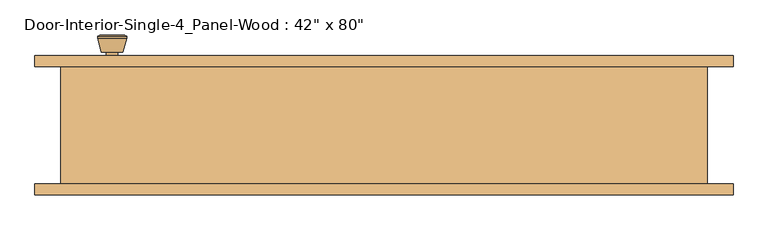
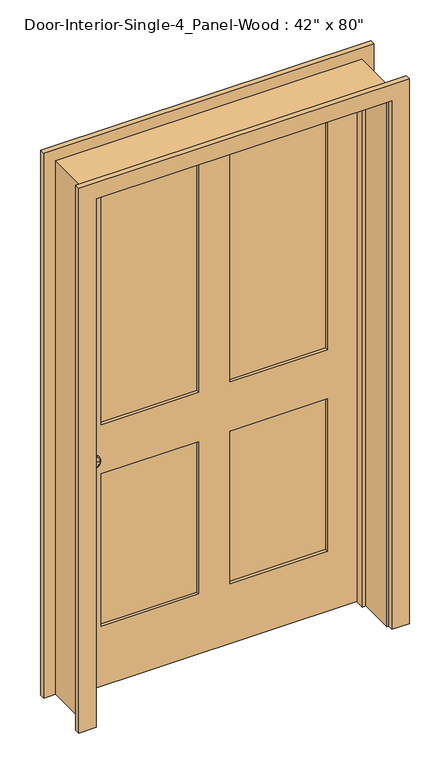
"""IFC4 building model written with IfcOpenShell, lengths in millimetres: door geometry."""

from ifc_helpers import new_model, si_unit, point, frame, frame_2d, origin, place, context, project, spatial, polyline, circle_curve, trimmed, segment, composite_curve, outline, extrude, faceted_brep, source, transform, mapped, element, save
from ifc_brep_helpers import plane_surface, cylinder_surface, revolved_surface, advanced_brep


def door_63baf7d0(model_context):
    return source(origin(), model_context, "Body", "SolidModel", [
        advanced_brep(
        [(-469.9, 57.5, 914.4), (-459.9, 57.5, 914.4), (-479.9, 57.5, 914.4), (-449.4241324, 8.5, 914.4), (-469.9, 8.5, 914.4), (-490.3758676, 8.5, 914.4), (-444.9, 10.3278681, 914.4), (-494.9, 10.3278681, 914.4), (-444.9, 13.7915463, 914.4), (-494.9, 13.7915463, 914.4), (-451.263764, 38.5, 914.4), (-488.536236, 38.5, 914.4), (-459.9, 38.5, 914.4), (-479.9, 38.5, 914.4)],
        [
            (0, 1),
            (1, 2, circle_curve(frame((-469.9, 57.5, 914.4), z_axis=(0.0, 1.0, 0.0), x_axis=(-1.0, 0.0, 0.0)), 10.0)),
            (2, 0),
            (2, 1, circle_curve(frame((-469.9, 57.5, 914.4), z_axis=(0.0, 1.0, 0.0), x_axis=(-1.0, 0.0, 0.0)), 10.0)),
            (3, 4),
            (4, 5),
            (5, 3, circle_curve(frame((-469.9, 8.5, 914.4), z_axis=(0.0, -1.0, 0.0), x_axis=(-1.0, 0.0, 0.0)), 20.4758676)),
            (3, 5, circle_curve(frame((-469.9, 8.5, 914.4), z_axis=(0.0, -1.0, 0.0), x_axis=(-1.0, 0.0, 0.0)), 20.4758676)),
            (6, 3),
            (5, 7),
            (7, 6, circle_curve(frame((-469.9, 10.3278681, 914.4), z_axis=(0.0, -1.0, 0.0), x_axis=(-1.0, 0.0, 0.0)), 25.0)),
            (6, 7, circle_curve(frame((-469.9, 10.3278681, 914.4), z_axis=(0.0, -1.0, 0.0), x_axis=(-1.0, 0.0, 0.0)), 25.0)),
            (8, 6),
            (7, 9),
            (9, 8, circle_curve(frame((-469.9, 13.7915463, 914.4), z_axis=(0.0, -1.0, 0.0), x_axis=(-1.0, 0.0, 0.0)), 25.0)),
            (8, 9, circle_curve(frame((-469.9, 13.7915463, 914.4), z_axis=(0.0, -1.0, 0.0), x_axis=(-1.0, 0.0, 0.0)), 25.0)),
            (10, 8),
            (9, 11),
            (11, 10, circle_curve(frame((-469.9, 38.5, 914.4), z_axis=(0.0, -1.0, 0.0), x_axis=(-1.0, 0.0, 0.0)), 18.636236)),
            (10, 11, circle_curve(frame((-469.9, 38.5, 914.4), z_axis=(0.0, -1.0, 0.0), x_axis=(-1.0, 0.0, 0.0)), 18.636236)),
            (12, 10),
            (11, 13),
            (13, 12, circle_curve(frame((-469.9, 38.5, 914.4), z_axis=(0.0, -1.0, 0.0), x_axis=(-1.0, 0.0, 0.0)), 10.0)),
            (12, 13, circle_curve(frame((-469.9, 38.5, 914.4), z_axis=(0.0, -1.0, 0.0), x_axis=(-1.0, 0.0, 0.0)), 10.0)),
            (1, 12),
            (13, 2),
        ],
        [
            plane_surface(frame((-469.9, 57.5, 914.4), z_axis=(0.0, 1.0, 0.0), x_axis=(-1.0, 0.0, 0.0))),
            plane_surface(frame((-469.9, 8.5, 914.4), z_axis=(0.0, -1.0, 0.0), x_axis=(-1.0, 0.0, 0.0))),
            revolved_surface(polyline([(-490.3758676, 8.5, 914.4), (-494.9, 10.3278681, 914.4)]), (-469.9, 57.5, 914.4), (0.0, 1.0, 0.0)),
            cylinder_surface(frame((-469.9, 57.5, 914.4), z_axis=(0.0, 1.0, 0.0), x_axis=(-1.0, 0.0, 0.0)), 25.0),
            revolved_surface(polyline([(-494.9, 13.7915463, 914.4), (-488.536236, 38.5, 914.4)]), (-469.9, 57.5, 914.4), (0.0, 1.0, 0.0)),
            plane_surface(frame((-469.9, 38.5, 914.4), z_axis=(0.0, 1.0, 0.0), x_axis=(-1.0, 0.0, 0.0))),
            cylinder_surface(frame((-469.9, 57.5, 914.4), z_axis=(0.0, 1.0, 0.0), x_axis=(-1.0, 0.0, 0.0)), 10.0),
        ],
        [
            (0, [[1, 2, 3]]),
            (0, [[-3, 4, -1]]),
            (1, [[5, 6, 7]]),
            (1, [[-6, -5, 8]]),
            (2, [[9, -7, 10, 11]]),
            (2, [[-10, -8, -9, 12]]),
            (3, [[13, -11, 14, 15]]),
            (3, [[-14, -12, -13, 16]]),
            (4, [[17, -15, 18, 19]]),
            (4, [[-18, -16, -17, 20]]),
            (5, [[21, -19, 22, 23]]),
            (5, [[-22, -20, -21, 24]]),
            (6, [[25, -23, 26, -2]]),
            (6, [[-26, -24, -25, -4]]),
        ],
    ),
        extrude(outline(composite_curve([segment(trimmed(circle_curve(frame_2d((914.4, -469.9)), 30.0), [point((914.4, -499.9))], [point((914.4, -439.9))], False, "CARTESIAN"), True, "CONTINUOUS"), segment(trimmed(circle_curve(frame_2d((914.4, -469.9)), 30.0), [point((914.4, -439.9))], [point((914.4, -499.9))], False, "CARTESIAN"), True, "CONTINUOUS")], self_intersect=False)), frame((0.0, 57.5, 0.0), z_axis=(0.0, 1.0, 0.0), x_axis=(0.0, 0.0, 1.0)), (0.0, 0.0, 1.0), 6.0),
        advanced_brep(
        [(-469.9, 104.425, 914.4), (-479.9, 104.425, 914.4), (-459.9, 104.425, 914.4), (-449.4241324, 153.425, 914.4), (-490.3758676, 153.425, 914.4), (-469.9, 153.425, 914.4), (-444.9, 151.5971319, 914.4), (-494.9, 151.5971319, 914.4), (-444.9, 148.1334537, 914.4), (-494.9, 148.1334537, 914.4), (-451.263764, 123.425, 914.4), (-488.536236, 123.425, 914.4), (-459.9, 123.425, 914.4), (-479.9, 123.425, 914.4)],
        [
            (0, 1),
            (1, 2, circle_curve(frame((-469.9, 104.425, 914.4), z_axis=(0.0, -1.0, 0.0), x_axis=(-1.0, 0.0, 0.0)), 10.0)),
            (2, 0),
            (2, 1, circle_curve(frame((-469.9, 104.425, 914.4), z_axis=(0.0, -1.0, 0.0), x_axis=(-1.0, 0.0, 0.0)), 10.0)),
            (3, 4, circle_curve(frame((-469.9, 153.425, 914.4), z_axis=(0.0, 1.0, 0.0), x_axis=(-1.0, 0.0, 0.0)), 20.4758676)),
            (4, 5),
            (5, 3),
            (4, 3, circle_curve(frame((-469.9, 153.425, 914.4), z_axis=(0.0, 1.0, 0.0), x_axis=(-1.0, 0.0, 0.0)), 20.4758676)),
            (6, 7, circle_curve(frame((-469.9, 151.5971319, 914.4), z_axis=(0.0, 1.0, 0.0), x_axis=(-1.0, 0.0, 0.0)), 25.0)),
            (7, 4),
            (3, 6),
            (7, 6, circle_curve(frame((-469.9, 151.5971319, 914.4), z_axis=(0.0, 1.0, 0.0), x_axis=(-1.0, 0.0, 0.0)), 25.0)),
            (8, 9, circle_curve(frame((-469.9, 148.1334537, 914.4), z_axis=(0.0, 1.0, 0.0), x_axis=(-1.0, 0.0, 0.0)), 25.0)),
            (9, 7),
            (6, 8),
            (9, 8, circle_curve(frame((-469.9, 148.1334537, 914.4), z_axis=(0.0, 1.0, 0.0), x_axis=(-1.0, 0.0, 0.0)), 25.0)),
            (10, 11, circle_curve(frame((-469.9, 123.425, 914.4), z_axis=(0.0, 1.0, 0.0), x_axis=(-1.0, 0.0, 0.0)), 18.636236)),
            (11, 9),
            (8, 10),
            (11, 10, circle_curve(frame((-469.9, 123.425, 914.4), z_axis=(0.0, 1.0, 0.0), x_axis=(-1.0, 0.0, 0.0)), 18.636236)),
            (12, 13, circle_curve(frame((-469.9, 123.425, 914.4), z_axis=(0.0, 1.0, 0.0), x_axis=(-1.0, 0.0, 0.0)), 10.0)),
            (13, 11),
            (10, 12),
            (13, 12, circle_curve(frame((-469.9, 123.425, 914.4), z_axis=(0.0, 1.0, 0.0), x_axis=(-1.0, 0.0, 0.0)), 10.0)),
            (1, 13),
            (12, 2),
        ],
        [
            plane_surface(frame((-469.9, 104.425, 914.4), z_axis=(0.0, -1.0, 0.0), x_axis=(-1.0, 0.0, 0.0))),
            plane_surface(frame((-469.9, 153.425, 914.4), z_axis=(0.0, 1.0, 0.0), x_axis=(-1.0, 0.0, 0.0))),
            revolved_surface(polyline([(-490.3758676, 153.425, 914.4), (-494.9, 151.5971319, 914.4)]), (-469.9, 104.425, 914.4), (0.0, -1.0, 0.0)),
            cylinder_surface(frame((-469.9, 104.425, 914.4), z_axis=(0.0, -1.0, 0.0), x_axis=(-1.0, 0.0, 0.0)), 25.0),
            revolved_surface(polyline([(-494.9, 148.1334537, 914.4), (-488.536236, 123.425, 914.4)]), (-469.9, 104.425, 914.4), (0.0, -1.0, 0.0)),
            plane_surface(frame((-469.9, 123.425, 914.4), z_axis=(0.0, -1.0, 0.0), x_axis=(-1.0, 0.0, 0.0))),
            cylinder_surface(frame((-469.9, 104.425, 914.4), z_axis=(0.0, -1.0, 0.0), x_axis=(-1.0, 0.0, 0.0)), 10.0),
        ],
        [
            (0, [[1, 2, 3]]),
            (0, [[-3, 4, -1]]),
            (1, [[5, 6, 7]]),
            (1, [[8, -7, -6]]),
            (2, [[9, 10, -5, 11]]),
            (2, [[12, -11, -8, -10]]),
            (3, [[13, 14, -9, 15]]),
            (3, [[16, -15, -12, -14]]),
            (4, [[17, 18, -13, 19]]),
            (4, [[20, -19, -16, -18]]),
            (5, [[21, 22, -17, 23]]),
            (5, [[24, -23, -20, -22]]),
            (6, [[-2, 25, -21, 26]]),
            (6, [[-4, -26, -24, -25]]),
        ],
    ),
        extrude(outline(composite_curve([segment(trimmed(circle_curve(frame_2d((914.4, -469.9)), 30.0), [point((914.4, -499.9))], [point((914.4, -439.9))], False, "CARTESIAN"), True, "CONTINUOUS"), segment(trimmed(circle_curve(frame_2d((914.4, -469.9)), 30.0), [point((914.4, -439.9))], [point((914.4, -499.9))], False, "CARTESIAN"), True, "CONTINUOUS")], self_intersect=False)), frame((0.0, 98.425, 0.0), z_axis=(0.0, 1.0, 0.0), x_axis=(0.0, 0.0, 1.0)), (0.0, 0.0, 1.0), 6.0),
        extrude(outline(polyline([(412.75, 75.1416667), (57.15, 75.1416667), (57.15, 86.7833333), (412.75, 86.7833333), (412.75, 75.1416667)])), frame((0.0, 0.0, 1009.65), z_axis=(0.0, 0.0, 1.0), x_axis=(1.0, 0.0, 0.0)), (0.0, 0.0, 1.0), 903.2875),
        extrude(outline(polyline([(-57.15, 75.1416667), (-412.75, 75.1416667), (-412.75, 86.7833333), (-57.15, 86.7833333), (-57.15, 75.1416667)])), frame((0.0, 0.0, 1009.65), z_axis=(0.0, 0.0, 1.0), x_axis=(1.0, 0.0, 0.0)), (0.0, 0.0, 1.0), 903.2875),
        extrude(outline(polyline([(412.75, 75.1416667), (57.15, 75.1416667), (57.15, 86.7833333), (412.75, 86.7833333), (412.75, 75.1416667)])), frame((0.0, 0.0, 231.775), z_axis=(0.0, 0.0, 1.0), x_axis=(1.0, 0.0, 0.0)), (0.0, 0.0, 1.0), 587.375),
        extrude(outline(polyline([(-57.15, 75.1416667), (-412.75, 75.1416667), (-412.75, 86.7833333), (-57.15, 86.7833333), (-57.15, 75.1416667)])), frame((0.0, 0.0, 231.775), z_axis=(0.0, 0.0, 1.0), x_axis=(1.0, 0.0, 0.0)), (0.0, 0.0, 1.0), 587.375),
        extrude(outline(polyline([(2032.0, -533.4), (0.0, -533.4), (0.0, 533.4), (2032.0, 533.4), (2032.0, -533.4)]), holes=[polyline([(1912.9375, 57.15), (1912.9375, 412.75), (1009.65, 412.75), (1009.65, 57.15), (1912.9375, 57.15)]), polyline([(1009.65, -57.15), (1009.65, -412.75), (1912.9375, -412.75), (1912.9375, -57.15), (1009.65, -57.15)]), polyline([(819.15, 57.15), (819.15, 412.75), (231.775, 412.75), (231.775, 57.15), (819.15, 57.15)]), polyline([(231.775, -57.15), (231.775, -412.75), (819.15, -412.75), (819.15, -57.15), (231.775, -57.15)])]), frame((0.0, 63.5, 0.0), z_axis=(0.0, 1.0, 0.0), x_axis=(0.0, 0.0, 1.0)), (0.0, 0.0, 1.0), 34.925),
        faceted_brep([(558.8, 98.425, 0.0), (558.8, -104.775, 0.0), (533.4, -104.775, 0.0), (533.4, 28.575, 0.0), (520.7, 28.575, 0.0), (520.7, 63.5, 0.0), (533.4, 63.5, 0.0), (533.4, 98.425, 0.0), (558.8, 98.425, 2057.4), (558.8, -104.775, 2057.4), (-558.8, -104.775, 2057.4), (-558.8, -104.775, 0.0), (-533.4, -104.775, 0.0), (-533.4, -104.775, 2032.0), (533.4, -104.775, 2032.0), (533.4, 28.575, 2032.0), (-533.4, 28.575, 2032.0), (-533.4, 28.575, 0.0), (-520.7, 28.575, 0.0), (-520.7, 28.575, 2019.3), (520.7, 28.575, 2019.3), (520.7, 63.5, 2019.3), (-520.7, 63.5, 2019.3), (-520.7, 63.5, 0.0), (-533.4, 63.5, 0.0), (-533.4, 63.5, 2032.0), (533.4, 63.5, 2032.0), (533.4, 98.425, 2032.0), (-533.4, 98.425, 2032.0), (-533.4, 98.425, 0.0), (-558.8, 98.425, 0.0), (-558.8, 98.425, 2057.4)], [[[0, 1, 2, 3, 4, 5, 6, 7]], [[1, 0, 8, 9]], [[2, 1, 9, 10, 11, 12, 13, 14]], [[3, 2, 14, 15]], [[4, 3, 15, 16, 17, 18, 19, 20]], [[5, 4, 20, 21]], [[6, 5, 21, 22, 23, 24, 25, 26]], [[7, 6, 26, 27]], [[0, 7, 27, 28, 29, 30, 31, 8]], [[9, 8, 31, 10]], [[15, 14, 13, 16]], [[21, 20, 19, 22]], [[27, 26, 25, 28]], [[30, 29, 24, 23, 18, 17, 12, 11]], [[10, 31, 30, 11]], [[16, 13, 12, 17]], [[22, 19, 18, 23]], [[28, 25, 24, 29]]]),
        extrude(outline(polyline([(0.0, 539.75), (0.0, 603.25), (2101.85, 603.25), (2101.85, -603.25), (0.0, -603.25), (0.0, -539.75), (2038.35, -539.75), (2038.35, 539.75), (0.0, 539.75)])), frame((0.0, -123.825, 0.0), z_axis=(0.0, 1.0, 0.0), x_axis=(0.0, 0.0, 1.0)), (0.0, 0.0, 1.0), 19.05),
        extrude(outline(polyline([(0.0, 539.75), (0.0, 603.25), (2101.85, 603.25), (2101.85, -603.25), (0.0, -603.25), (0.0, -539.75), (2038.35, -539.75), (2038.35, 539.75), (0.0, 539.75)])), frame((0.0, 98.425, 0.0), z_axis=(0.0, 1.0, 0.0), x_axis=(0.0, 0.0, 1.0)), (0.0, 0.0, 1.0), 19.05),
    ])


if __name__ == "__main__":
    model = new_model("IFC4")
    model_context = context("Model", 3, world=origin())
    ifc_project = project(units=[si_unit("LENGTHUNIT", "METRE", prefix="MILLI")], contexts=[model_context])
    site = spatial("IfcSite", under=ifc_project)
    building = spatial("IfcBuilding", under=site)
    placement = place(None, origin())
    door_shape = door_63baf7d0(model_context)
    element("IfcDoor", 1, ObjectType="Door-Interior-Single-4_Panel-Wood : 42\" x 80\"", at=placement, inside=building, context=model_context, shape_type="MappedRepresentation", body=[
        mapped(door_shape, transform((0.0, 0.0, 0.0), x_axis=(1.0, 0.0, 0.0), y_axis=(0.0, 1.0, 0.0), z_axis=(0.0, 0.0, 1.0))),
    ])
    save(model, "model.ifc")

# Revit data of these elements
# Type "Door-Interior-Single-4_Panel-Wood : 42\" x 80\""
#   Type Mark = "20"
#   Assembly Code = "C1020300"
#   Analytic Construction = "Wooden"
#   Top Rail = 0' - 4 11/16"
#   Thickness = 0' - 1 3/8"
#   Thermal Resistance (R) = 2.5876 (h·ft²·°F)/BTU
#   Swing Angle [instance default] = 90.00°
#   Stiles = 0' - 4 3/4"
#   Rough Width = 3' - 8"
#   Rough Height = 6' - 9"
#   Mullion = 0' - 4 1/2"
#   Lock Rail = 0' - 7 1/2"
#   Height = 6' - 8"
#   Width = 3' - 6"
#   Heat Transfer Coefficient (U) = 0.3865 BTU/(h·ft²·°F)
#   Bottom Rail = 0' - 9 1/8"
#   Trim Material = Cherry
#   Panel Material = Cherry
#   Frame Material = Cherry
#   Door Handle Material = Aluminum
#   Visual Light Transmittance = 0
#   Solar Heat Gain Coefficient = 0
#   Wall Closure = (empty or 0)
#   Function = (empty or 0)
# Element 1 (IfcDoor, "Door-Interior-Single-4_Panel-Wood : 42\" x 80\"")
#   Materials on its faces: "Cherry", "Aluminum"
# Materials
#   "Cherry": class "Wood", colour RGB 226 177 128, transparency 0, Description = "Prunus Serotina", Cost = 0
#   "Aluminum": class "Metal", colour RGB 247 247 247, transparency 0, Description = "Aluminum 6061", Cost = 0
